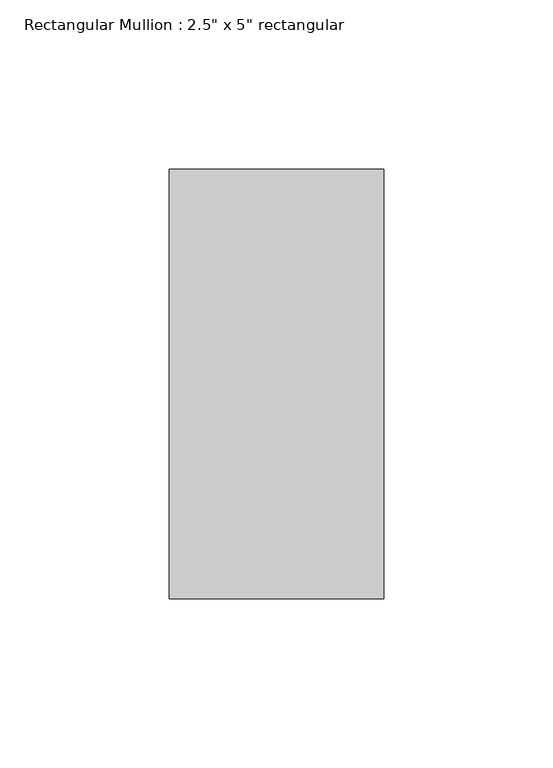
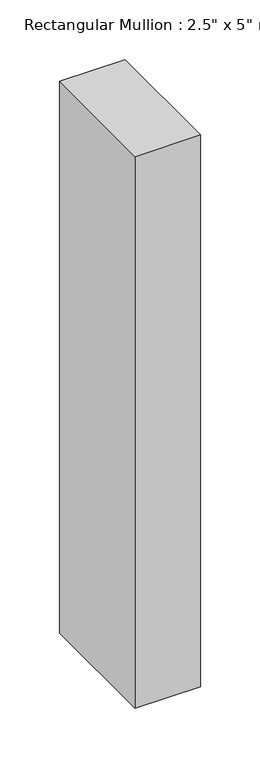
"""IFC4 building model written with IfcOpenShell, lengths in millimetres: member geometry."""

from ifc_helpers import new_model, si_unit, frame, origin, place, context, project, spatial, polyline, outline, extrude, source, transform, mapped, element, save


def member_6103f85b(model_context):
    return source(origin(), model_context, "Body", "SweptSolid", [
        extrude(outline(polyline([(31.75, 63.5), (31.75, -63.5), (-31.75, -63.5), (-31.75, 63.5), (31.75, 63.5)])), frame((0.0, 0.0, -565.15), z_axis=(0.0, 0.0, 1.0), x_axis=(1.0, 0.0, 0.0)), (0.0, 0.0, 1.0), 565.15),
    ])


if __name__ == "__main__":
    model = new_model("IFC4")
    model_context = context("Model", 3, world=origin())
    ifc_project = project(units=[si_unit("LENGTHUNIT", "METRE", prefix="MILLI")], contexts=[model_context])
    site = spatial("IfcSite", under=ifc_project)
    building = spatial("IfcBuilding", under=site)
    placement = place(None, origin())
    member_shape = member_6103f85b(model_context)
    element("IfcMember", 1, ObjectType="Rectangular Mullion : 2.5\" x 5\" rectangular", at=placement, inside=building, context=model_context, shape_type="MappedRepresentation", body=[
        mapped(member_shape, transform((0.0, 0.0, 0.0), x_axis=(1.0, 0.0, 0.0), y_axis=(0.0, 1.0, 0.0), z_axis=(0.0, 0.0, 1.0))),
    ])
    save(model, "model.ifc")

# Revit data of these elements
# Type "Rectangular Mullion : 2.5\" x 5\" rectangular"
#   built-in parameter 1007304 = 0.416667 (stored number, unit not read)
#   built-in parameter 1007301 = 0.104167 (stored number, unit not read)
#   built-in parameter 1007300 = 0.104167 (stored number, unit not read)
